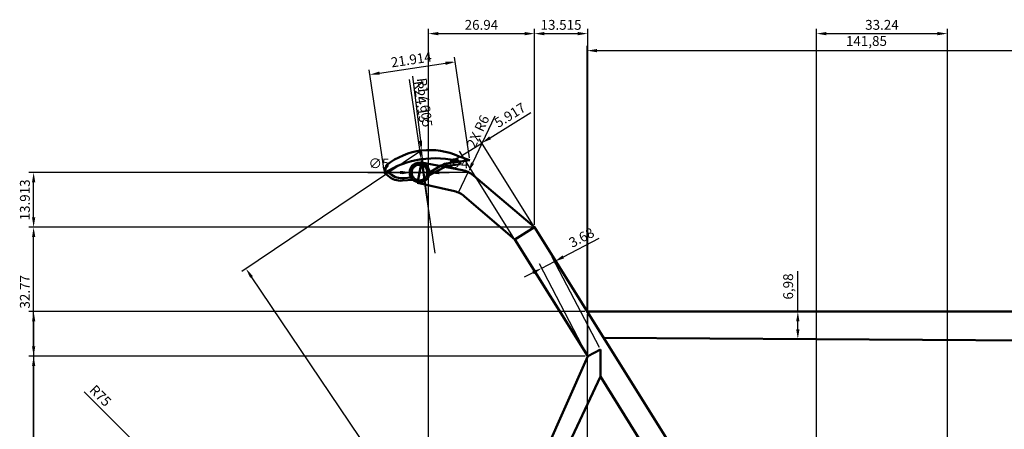
# Model space of a CAD drawing. Units: millimetres. Extents: x 1068 to 1546, y 1743 to 2032.
# Tile 5 of 9: x 1068 to 1318, y 1928 to 2032. Entities that reach past the tile are written whole.
import ezdxf

# ---------------------------------------------------------------- set-up
doc = ezdxf.new("R2010")
doc.units = ezdxf.units.MM
doc.layers.add('M-DIMS', color=2, linetype='Continuous', lineweight=25)
doc.layers.add('M-OUTL', color=7, linetype='Continuous', lineweight=50)
doc.styles.get("Standard").update_dxf_attribs({"font": 'arial.ttf'})
doc.dimstyles.new('ISO-25', dxfattribs={"dimtxt": 2.5, "dimasz": 2.5, "dimexe": 1.25, "dimexo": 0.625, "dimtad": 1, "dimtxsty": 'Standard', "dimcen": 2.5, "dimadec": 0, "dimazin": 0, "dimtfac": 1, "dimtmove": 0, "dimatfit": 3, "dimfxl": 1, "dimarcsym": 0})

# ---------------------------------------------------------------- blocks, each defined once
blk = doc.blocks.new('*D21')
at = {"layer": 'Defpoints', "color": 0, "transparency": 16777216}
for p in [(1266.05, 1957.56), (1267.8, 1957.56), (1267.8, 1950.59)]:
    blk.add_point(p, dxfattribs=at)
at = {"layer": 'M-DIMS', "color": 0, "lineweight": -2, "transparency": 16777216}
for p, q in [((1266.05, 1957.56), (1266.05, 1967.82)), ((1267.18, 1957.56), (1264.8, 1957.56)), ((1266.05, 1953.09), (1266.05, 1955.06)), ((1267.18, 1950.59), (1264.8, 1950.59))]:
    blk.add_line(p, q, dxfattribs=at)
at = {"layer": 'M-DIMS', "color": 0, "transparency": 16777216}
for points in [[(1265.63, 1955.06), (1266.47, 1955.06), (1266.05, 1957.56)], [(1265.63, 1953.09), (1266.47, 1953.09), (1266.05, 1950.59)]]:
    blk.add_solid(points, dxfattribs=at)
at = {"layer": 'M-DIMS', "color": 0, "transparency": 16777216, "insert": (1263.92, 1963.94), "char_height": 2.5, "attachment_point": 5, "rotation": 90}
blk.add_mtext('6,98', dxfattribs=at)
blk = doc.blocks.new('*D22')
at = {"layer": 'Defpoints', "color": 0, "transparency": 16777216}
for p in [(1354.41, 2023.87), (1212.56, 1957.56), (1354.41, 1957.56)]:
    blk.add_point(p, dxfattribs=at)
at = {"layer": 'M-DIMS', "color": 0, "lineweight": -2, "transparency": 16777216}
for p, q in [((1212.56, 1958.19), (1212.56, 2025.12)), ((1215.06, 2023.87), (1351.91, 2023.87)), ((1354.41, 1958.19), (1354.41, 2025.12))]:
    blk.add_line(p, q, dxfattribs=at)
at = {"layer": 'M-DIMS', "color": 0, "transparency": 16777216}
for points in [[(1215.06, 2024.29), (1215.06, 2023.46), (1212.56, 2023.87)], [(1351.91, 2024.29), (1351.91, 2023.46), (1354.41, 2023.87)]]:
    blk.add_solid(points, dxfattribs=at)
at = {"layer": 'M-DIMS', "color": 0, "transparency": 16777216, "insert": (1283.48, 2026), "char_height": 2.5, "attachment_point": 5}
blk.add_mtext('141,85', dxfattribs=at)
blk = doc.blocks.new('*D23')
at = {"layer": 'Defpoints', "color": 0, "transparency": 16777216}
for p in [(1170.51, 1998.5), (1125.92, 1968.44), (1270.79, 1849.76)]:
    blk.add_point(p, dxfattribs=at)
at = {"layer": 'M-DIMS', "color": 0, "lineweight": -2, "transparency": 16777216}
for p, q in [((1169.99, 1998.15), (1124.89, 1967.74)), ((1224.8, 1821.77), (1127.32, 1966.36)), ((1270.27, 1849.41), (1225.16, 1819))]:
    blk.add_line(p, q, dxfattribs=at)
at = {"layer": 'M-DIMS', "color": 0, "transparency": 16777216}
for points in [[(1127.67, 1966.6), (1126.98, 1966.13), (1125.92, 1968.44)], [(1225.15, 1822.01), (1224.45, 1821.54), (1226.2, 1819.7)]]:
    blk.add_solid(points, dxfattribs=at)
at = {"layer": 'M-DIMS', "color": 0, "transparency": 16777216, "insert": (1177.82, 1895.26), "char_height": 2.5, "attachment_point": 5, "rotation": 303.9872}
blk.add_mtext('179,38', dxfattribs=at)
blk = doc.blocks.new('*D26')
at = {"layer": 'Defpoints', "color": 0, "transparency": 16777216}
for p in [(1304.02, 2028.2), (1270.79, 1849.76), (1304.02, 1849.7)]:
    blk.add_point(p, dxfattribs=at)
at = {"layer": 'M-DIMS', "color": 0, "lineweight": -2, "transparency": 16777216}
for p, q in [((1270.79, 1850.39), (1270.79, 2029.45)), ((1273.29, 2028.2), (1301.52, 2028.2)), ((1304.02, 1850.33), (1304.02, 2029.45))]:
    blk.add_line(p, q, dxfattribs=at)
at = {"layer": 'M-DIMS', "color": 0, "transparency": 16777216}
for points in [[(1273.29, 2028.61), (1273.29, 2027.78), (1270.79, 2028.2)], [(1301.52, 2028.61), (1301.52, 2027.78), (1304.02, 2028.2)]]:
    blk.add_solid(points, dxfattribs=at)
at = {"layer": 'M-DIMS', "color": 0, "transparency": 16777216, "insert": (1287.41, 2030.1), "char_height": 2.5, "attachment_point": 5}
blk.add_mtext('33.24', dxfattribs=at)
blk = doc.blocks.new('*D28')
at = {"layer": 'Defpoints', "color": 0, "transparency": 16777216}
for p in [(1071.98, 1946.21), (1212.68, 1946.21), (1172.23, 1849.76)]:
    blk.add_point(p, dxfattribs=at)
at = {"layer": 'M-DIMS', "color": 0, "lineweight": -2, "transparency": 16777216}
for p, q in [((1212.06, 1946.21), (1070.73, 1946.21)), ((1071.98, 1852.26), (1071.98, 1943.71)), ((1171.6, 1849.76), (1070.73, 1849.76))]:
    blk.add_line(p, q, dxfattribs=at)
at = {"layer": 'M-DIMS', "color": 0, "transparency": 16777216}
for points in [[(1071.57, 1943.71), (1072.4, 1943.71), (1071.98, 1946.21)], [(1071.57, 1852.26), (1072.4, 1852.26), (1071.98, 1849.76)]]:
    blk.add_solid(points, dxfattribs=at)
at = {"layer": 'M-DIMS', "color": 0, "transparency": 16777216, "insert": (1070.08, 1897.98), "char_height": 2.5, "attachment_point": 5, "rotation": 90}
blk.add_mtext('96.44', dxfattribs=at)
blk = doc.blocks.new('*D29')
at = {"layer": 'Defpoints', "color": 0, "transparency": 16777216}
for p in [(1071.98, 1978.98), (1199.17, 1978.98), (1212.68, 1946.21)]:
    blk.add_point(p, dxfattribs=at)
at = {"layer": 'M-DIMS', "color": 0, "lineweight": -2, "transparency": 16777216}
for p, q in [((1198.54, 1978.98), (1070.73, 1978.98)), ((1071.98, 1948.71), (1071.98, 1976.48)), ((1212.06, 1946.21), (1070.73, 1946.21))]:
    blk.add_line(p, q, dxfattribs=at)
at = {"layer": 'M-DIMS', "color": 0, "transparency": 16777216}
for points in [[(1071.57, 1976.48), (1072.4, 1976.48), (1071.98, 1978.98)], [(1071.57, 1948.71), (1072.4, 1948.71), (1071.98, 1946.21)]]:
    blk.add_solid(points, dxfattribs=at)
at = {"layer": 'M-DIMS', "color": 0, "transparency": 16777216, "insert": (1070.08, 1962.59), "char_height": 2.5, "attachment_point": 5, "rotation": 90}
blk.add_mtext('32.77', dxfattribs=at)
blk = doc.blocks.new('*D30')
at = {"layer": 'Defpoints', "color": 0, "transparency": 16777216}
for p in [(1071.98, 1992.89), (1169.99, 1992.89), (1199.17, 1978.98)]:
    blk.add_point(p, dxfattribs=at)
at = {"layer": 'M-DIMS', "color": 0, "lineweight": -2, "transparency": 16777216}
for p, q in [((1169.36, 1992.89), (1070.73, 1992.89)), ((1071.98, 1981.48), (1071.98, 1990.39)), ((1198.54, 1978.98), (1070.73, 1978.98))]:
    blk.add_line(p, q, dxfattribs=at)
at = {"layer": 'M-DIMS', "color": 0, "transparency": 16777216}
for points in [[(1071.57, 1990.39), (1072.4, 1990.39), (1071.98, 1992.89)], [(1071.57, 1981.48), (1072.4, 1981.48), (1071.98, 1978.98)]]:
    blk.add_solid(points, dxfattribs=at)
at = {"layer": 'M-DIMS', "color": 0, "transparency": 16777216, "insert": (1070.08, 1985.94), "char_height": 2.5, "attachment_point": 5, "rotation": 90}
blk.add_mtext('13.913', dxfattribs=at)
blk = doc.blocks.new('*D31')
at = {"layer": 'Defpoints', "color": 0, "transparency": 16777216}
for p in [(1199.17, 2028.2), (1199.17, 1978.98), (1172.23, 1849.76)]:
    blk.add_point(p, dxfattribs=at)
at = {"layer": 'M-DIMS', "color": 0, "lineweight": -2, "transparency": 16777216}
for p, q in [((1172.23, 1850.39), (1172.23, 2029.45)), ((1174.73, 2028.2), (1196.67, 2028.2)), ((1199.17, 1979.6), (1199.17, 2029.45))]:
    blk.add_line(p, q, dxfattribs=at)
at = {"layer": 'M-DIMS', "color": 0, "transparency": 16777216}
for points in [[(1174.73, 2028.61), (1174.73, 2027.78), (1172.23, 2028.2)], [(1196.67, 2028.61), (1196.67, 2027.78), (1199.17, 2028.2)]]:
    blk.add_solid(points, dxfattribs=at)
at = {"layer": 'M-DIMS', "color": 0, "transparency": 16777216, "insert": (1185.7, 2030.1), "char_height": 2.5, "attachment_point": 5}
blk.add_mtext('26.94', dxfattribs=at)
blk = doc.blocks.new('*D32')
at = {"layer": 'Defpoints', "color": 0, "transparency": 16777216}
for p in [(1212.68, 2028.2), (1199.17, 1978.98), (1212.68, 1946.21)]:
    blk.add_point(p, dxfattribs=at)
at = {"layer": 'M-DIMS', "color": 0, "lineweight": -2, "transparency": 16777216}
for p, q in [((1199.17, 1979.6), (1199.17, 2029.45)), ((1201.67, 2028.2), (1210.18, 2028.2)), ((1212.68, 1946.83), (1212.68, 2029.45))]:
    blk.add_line(p, q, dxfattribs=at)
at = {"layer": 'M-DIMS', "color": 0, "transparency": 16777216}
for points in [[(1201.67, 2028.61), (1201.67, 2027.78), (1199.17, 2028.2)], [(1210.18, 2028.61), (1210.18, 2027.78), (1212.68, 2028.2)]]:
    blk.add_solid(points, dxfattribs=at)
at = {"layer": 'M-DIMS', "color": 0, "transparency": 16777216, "insert": (1205.92, 2030.1), "char_height": 2.5, "attachment_point": 5}
blk.add_mtext('13.515', dxfattribs=at)
blk = doc.blocks.new('*D33')
at = {"layer": 'Defpoints', "color": 0, "transparency": 16777216}
for p in [(1179.05, 2021.02), (1182.77, 1996.04), (1161.1, 1992.81)]:
    blk.add_point(p, dxfattribs=at)
at = {"layer": 'M-DIMS', "color": 0, "lineweight": -2, "transparency": 16777216}
for p, q in [((1159.84, 2018.15), (1176.57, 2020.65)), ((1182.68, 1996.66), (1178.86, 2022.25)), ((1161.01, 1993.43), (1157.19, 2019.02))]:
    blk.add_line(p, q, dxfattribs=at)
at = {"layer": 'M-DIMS', "color": 0, "transparency": 16777216}
for points in [[(1176.51, 2021.06), (1176.63, 2020.24), (1179.05, 2021.02)], [(1159.78, 2018.56), (1159.91, 2017.74), (1157.37, 2017.78)]]:
    blk.add_solid(points, dxfattribs=at)
at = {"layer": 'M-DIMS', "color": 0, "transparency": 16777216, "insert": (1167.93, 2021.28), "char_height": 2.5, "attachment_point": 5, "rotation": 8.4889}
blk.add_mtext('21.914', dxfattribs=at)
blk = doc.blocks.new('*D41')
at = {"layer": 'Defpoints', "color": 0, "transparency": 16777216}
for p in [(1185.78, 2000.39), (1199.17, 1978.98), (1194.15, 1975.84)]:
    blk.add_point(p, dxfattribs=at)
at = {"layer": 'M-DIMS', "color": 0, "lineweight": -2, "transparency": 16777216}
for p, q in [((1187.9, 2001.71), (1198.23, 2008.18)), ((1180.76, 1997.25), (1185.78, 2000.39)), ((1198.83, 1979.51), (1185.12, 2001.45)), ((1193.82, 1976.37), (1180.1, 1998.31)), ((1178.64, 1995.93), (1176.52, 1994.6))]:
    blk.add_line(p, q, dxfattribs=at)
at = {"layer": 'M-DIMS', "color": 0, "transparency": 16777216}
for points in [[(1187.68, 2002.07), (1188.12, 2001.36), (1185.78, 2000.39)], [(1178.42, 1996.28), (1178.86, 1995.57), (1180.76, 1997.25)]]:
    blk.add_solid(points, dxfattribs=at)
at = {"layer": 'M-DIMS', "color": 0, "transparency": 16777216, "insert": (1193.12, 2007.22), "char_height": 2.5, "attachment_point": 5, "rotation": 32.0179}
blk.add_mtext('5.917', dxfattribs=at)
blk = doc.blocks.new('*D44')
at = {"layer": 'Defpoints', "color": 0, "transparency": 16777216}
for p in [(1204.28, 1970.3), (1215.95, 1947.91), (1212.68, 1946.21)]:
    blk.add_point(p, dxfattribs=at)
at = {"layer": 'M-DIMS', "color": 0, "lineweight": -2, "transparency": 16777216}
for p, q in [((1206.5, 1971.46), (1215.58, 1976.19)), ((1215.66, 1948.46), (1203.7, 1971.41)), ((1212.39, 1946.76), (1200.43, 1969.71)), ((1201.01, 1968.6), (1204.28, 1970.3)), ((1198.79, 1967.44), (1196.58, 1966.29))]:
    blk.add_line(p, q, dxfattribs=at)
at = {"layer": 'M-DIMS', "color": 0, "transparency": 16777216}
for points in [[(1206.3, 1971.83), (1206.69, 1971.09), (1204.28, 1970.3)], [(1198.6, 1967.81), (1198.99, 1967.07), (1201.01, 1968.6)]]:
    blk.add_solid(points, dxfattribs=at)
at = {"layer": 'M-DIMS', "color": 0, "transparency": 16777216, "insert": (1211.27, 1976.09), "char_height": 2.5, "attachment_point": 5, "rotation": 27.5268}
blk.add_mtext('3.68', dxfattribs=at)
blk = doc.blocks.new('*D45')
at = {"layer": 'Defpoints', "color": 0, "transparency": 16777216}
for p in [(1212.56, 1957.56), (1273.55, 1860.03), (1273.55, 1744.51)]:
    blk.add_point(p, dxfattribs=at)
at = {"layer": 'M-DIMS', "color": 0, "lineweight": -2, "transparency": 16777216}
for p, q in [((1212.56, 1956.94), (1212.56, 1743.26)), ((1273.55, 1859.4), (1273.55, 1743.26)), ((1215.06, 1744.51), (1271.05, 1744.51))]:
    blk.add_line(p, q, dxfattribs=at)
at = {"layer": 'M-DIMS', "color": 0, "transparency": 16777216}
for points in [[(1215.06, 1744.93), (1215.06, 1744.1), (1212.56, 1744.51)], [(1271.05, 1744.93), (1271.05, 1744.1), (1273.55, 1744.51)]]:
    blk.add_solid(points, dxfattribs=at)
at = {"layer": 'M-DIMS', "color": 0, "transparency": 16777216, "insert": (1243.05, 1746.41), "char_height": 2.5, "attachment_point": 5}
blk.add_mtext('60.99', dxfattribs=at)
blk = doc.blocks.new('*D46')
at = {"layer": 'Defpoints', "color": 0, "transparency": 16777216}
for p in [(1212.56, 1957.56), (1071.98, 1860.03), (1273.55, 1860.03)]:
    blk.add_point(p, dxfattribs=at)
at = {"layer": 'M-DIMS', "color": 0, "lineweight": -2, "transparency": 16777216}
for p, q in [((1211.93, 1957.56), (1070.73, 1957.56)), ((1071.98, 1955.06), (1071.98, 1862.53)), ((1272.92, 1860.03), (1070.73, 1860.03))]:
    blk.add_line(p, q, dxfattribs=at)
at = {"layer": 'M-DIMS', "color": 0, "transparency": 16777216}
for points in [[(1071.57, 1955.06), (1072.4, 1955.06), (1071.98, 1957.56)], [(1071.57, 1862.53), (1072.4, 1862.53), (1071.98, 1860.03)]]:
    blk.add_solid(points, dxfattribs=at)
at = {"layer": 'M-DIMS', "color": 0, "transparency": 16777216, "insert": (1070.08, 1908.79), "char_height": 2.5, "attachment_point": 5, "rotation": 90}
blk.add_mtext('97.53', dxfattribs=at)
blk = doc.blocks.new('*D47')
at = {"layer": 'Defpoints', "color": 0, "transparency": 16777216}
for p in [(1361.34, 1946.14), (1282.2, 1868.65), (1361.34, 1744.51)]:
    blk.add_point(p, dxfattribs=at)
at = {"layer": 'M-DIMS', "color": 0, "lineweight": -2, "transparency": 16777216}
for p, q in [((1361.34, 1945.51), (1361.34, 1743.26)), ((1282.2, 1868.03), (1282.2, 1743.26)), ((1284.7, 1744.51), (1358.84, 1744.51))]:
    blk.add_line(p, q, dxfattribs=at)
at = {"layer": 'M-DIMS', "color": 0, "transparency": 16777216}
for points in [[(1284.7, 1744.93), (1284.7, 1744.1), (1282.2, 1744.51)], [(1358.84, 1744.93), (1358.84, 1744.1), (1361.34, 1744.51)]]:
    blk.add_solid(points, dxfattribs=at)
at = {"layer": 'M-DIMS', "color": 0, "transparency": 16777216, "insert": (1321.77, 1746.41), "char_height": 2.5, "attachment_point": 5}
blk.add_mtext('79.14', dxfattribs=at)
blk = doc.blocks.new('*D48')
at = {"layer": 'Defpoints', "color": 0, "transparency": 16777216}
for p in [(1361.34, 1946.14), (1507.48, 1946.14), (1282.2, 1868.65)]:
    blk.add_point(p, dxfattribs=at)
at = {"layer": 'M-DIMS', "color": 0, "lineweight": -2, "transparency": 16777216}
for p, q in [((1361.96, 1946.14), (1508.73, 1946.14)), ((1507.48, 1871.15), (1507.48, 1943.64)), ((1282.82, 1868.65), (1508.73, 1868.65))]:
    blk.add_line(p, q, dxfattribs=at)
at = {"layer": 'M-DIMS', "color": 0, "transparency": 16777216}
for points in [[(1507.06, 1943.64), (1507.89, 1943.64), (1507.48, 1946.14)], [(1507.06, 1871.15), (1507.89, 1871.15), (1507.48, 1868.65)]]:
    blk.add_solid(points, dxfattribs=at)
at = {"layer": 'M-DIMS', "color": 0, "transparency": 16777216, "insert": (1505.58, 1907.39), "char_height": 2.5, "attachment_point": 5, "rotation": 90}
blk.add_mtext('77.49', dxfattribs=at)
blk = doc.blocks.new('*D57')
at = {"layer": 'Defpoints', "color": 0, "transparency": 16777216}
for p in [(1119.2, 1902.8), (1172.23, 1849.76)]:
    blk.add_point(p, dxfattribs=at)
at = {"layer": 'M-DIMS', "color": 0, "lineweight": -2, "transparency": 16777216}
for p, q in [((1084.82, 1937.18), (1117.43, 1904.57)), ((1172.23, 1849.76), (1119.2, 1902.8))]:
    blk.add_line(p, q, dxfattribs=at)
at = {"layer": 'M-DIMS', "color": 0, "transparency": 16777216}
blk.add_solid([(1117.73, 1904.86), (1117.14, 1904.27), (1119.2, 1902.8)], dxfattribs=at)
at = {"layer": 'M-DIMS', "color": 0, "transparency": 16777216, "insert": (1088.72, 1935.96), "char_height": 2.5, "attachment_point": 5, "rotation": 314.9948}
blk.add_mtext('R75', dxfattribs=at)
blk = doc.blocks.new('*D65')
at = {"layer": 'Defpoints', "color": 0, "transparency": 16777216}
for p in [(1170.38, 1996.26), (1173.97, 1972.4)]:
    blk.add_point(p, dxfattribs=at)
at = {"layer": 'M-DIMS', "color": 0, "lineweight": -2, "transparency": 16777216}
for p, q in [((1167.32, 2016.55), (1170, 1998.73)), ((1173.97, 1972.4), (1170.38, 1996.26))]:
    blk.add_line(p, q, dxfattribs=at)
at = {"layer": 'M-DIMS', "color": 0, "transparency": 16777216}
blk.add_solid([(1170.42, 1998.79), (1169.59, 1998.67), (1170.38, 1996.26)], dxfattribs=at)
at = {"layer": 'M-DIMS', "color": 0, "transparency": 16777216, "insert": (1170.1, 2010.86), "char_height": 2.5, "attachment_point": 5, "rotation": 278.5724}
blk.add_mtext('R24.13', dxfattribs=at)
blk = doc.blocks.new('*D66')
at = {"layer": 'Defpoints', "color": 0, "transparency": 16777216}
for p in [(1170.51, 1998.5), (1172.63, 1981.02)]:
    blk.add_point(p, dxfattribs=at)
at = {"layer": 'M-DIMS', "color": 0, "lineweight": -2, "transparency": 16777216}
for p, q in [((1168.22, 2017.4), (1170.21, 2000.98)), ((1172.63, 1981.02), (1170.51, 1998.5))]:
    blk.add_line(p, q, dxfattribs=at)
at = {"layer": 'M-DIMS', "color": 0, "transparency": 16777216}
blk.add_solid([(1170.63, 2001.03), (1169.8, 2000.93), (1170.51, 1998.5)], dxfattribs=at)
at = {"layer": 'M-DIMS', "color": 0, "transparency": 16777216, "insert": (1170.95, 2010.66), "char_height": 2.5, "attachment_point": 5, "rotation": 276.9175}
blk.add_mtext('R17.605', dxfattribs=at)
blk = doc.blocks.new('*D76')
at = {"layer": 'Defpoints', "color": 0, "transparency": 16777216}
for p in [(1182.37, 1993.03), (1179.78, 1987.62)]:
    blk.add_point(p, dxfattribs=at)
at = {"layer": 'M-DIMS', "color": 0, "lineweight": -2, "transparency": 16777216}
for p, q in [((1189.13, 2007.19), (1183.44, 1995.29)), ((1179.78, 1987.62), (1182.37, 1993.03))]:
    blk.add_line(p, q, dxfattribs=at)
at = {"layer": 'M-DIMS', "color": 0, "transparency": 16777216}
blk.add_solid([(1183.07, 1995.47), (1183.82, 1995.11), (1182.37, 1993.03)], dxfattribs=at)
at = {"layer": 'M-DIMS', "color": 0, "transparency": 16777216, "insert": (1185.11, 2003.19), "char_height": 2.5, "attachment_point": 5, "rotation": 64.4837}
blk.add_mtext('2X R6', dxfattribs=at)
blk = doc.blocks.new('*D79')
at = {"layer": 'Defpoints', "color": 0, "transparency": 16777216}
for p in [(1167.49, 1992.9), (1172.49, 1992.89)]:
    blk.add_point(p, dxfattribs=at)
at = {"layer": 'M-DIMS', "color": 0, "lineweight": -2, "transparency": 16777216}
for p, q in [((1156.86, 1992.93), (1164.99, 1992.91)), ((1172.49, 1992.89), (1167.49, 1992.9)), ((1174.99, 1992.88), (1177.49, 1992.87))]:
    blk.add_line(p, q, dxfattribs=at)
at = {"layer": 'M-DIMS', "color": 0, "transparency": 16777216}
for points in [[(1164.99, 1993.32), (1164.98, 1992.49), (1167.49, 1992.9)], [(1174.99, 1993.29), (1174.98, 1992.46), (1172.49, 1992.89)]]:
    blk.add_solid(points, dxfattribs=at)
at = {"layer": 'M-DIMS', "color": 0, "transparency": 16777216, "insert": (1159.68, 1994.89), "char_height": 2.5, "attachment_point": 5, "rotation": 359.8328}
blk.add_mtext('∅5', dxfattribs=at)
blk = doc.blocks.new('*D80')
at = {"layer": 'Defpoints', "color": 0, "transparency": 16777216}
for p in [(1167.99, 1992.89), (1171.99, 1992.9)]:
    blk.add_point(p, dxfattribs=at)
at = {"layer": 'M-DIMS', "color": 0, "lineweight": -2, "transparency": 16777216}
for p, q in [((1165.49, 1992.88), (1162.99, 1992.87)), ((1167.99, 1992.89), (1171.99, 1992.9)), ((1182.58, 1992.94), (1174.49, 1992.91))]:
    blk.add_line(p, q, dxfattribs=at)
at = {"layer": 'M-DIMS', "color": 0, "transparency": 16777216}
for points in [[(1165.48, 1993.29), (1165.49, 1992.46), (1167.99, 1992.89)], [(1174.48, 1993.33), (1174.49, 1992.49), (1171.99, 1992.9)]]:
    blk.add_solid(points, dxfattribs=at)
at = {"layer": 'M-DIMS', "color": 0, "transparency": 16777216, "insert": (1179.78, 1994.9), "char_height": 2.5, "attachment_point": 5, "rotation": 0.2063}
blk.add_mtext('∅4', dxfattribs=at)

msp = doc.modelspace()

# ---------------------------------------------------------------- linework, layer by layer
at = {"layer": 'M-OUTL'}
for p, q in [((1169.5051, 1990.3234), (1170.4659, 1995.4621)), ((1180.8842, 1993.5142), (1170.4486, 1995.4653)), ((1177.3514, 1995.2964), (1180.2594, 1995.6971)), ((1182.7731, 1996.0435), (1180.0358, 1996.9929)), ((1180.2594, 1995.6971), (1182.7731, 1996.0435)), ((1180.2594, 1995.6971), (1180.3491, 1995.0462)), ((1161.0994, 1992.8087), (1161.6258, 1994.7591)), ((1161.7904, 1993.15), (1161.0994, 1992.8087)), ((1162.5033, 1992.5661), (1161.7904, 1993.15)), ((1176.1114, 1994.1402), (1172.3597, 1992.1098)), ((1172.4855, 1992.8927), (1175.5122, 1994.6606)), ((1180.3491, 1995.0462), (1177.8086, 1994.6961)), ((1162.0058, 1992.028), (1161.0994, 1992.8087)), ((1168.3037, 1991.043), (1165.6669, 1990.8324)), ((1167.8411, 1991.6077), (1166.1159, 1991.4538)), ((1168.3037, 1991.043), (1168.3037, 1991.043)), ((1199.166, 1978.9798), (1183.6733, 1992.1831)), ((1178.8506, 1988.1569), (1169.5051, 1990.3234)), ((1194.1495, 1975.8429), (1181.4201, 1986.8504)), ((1194.1495, 1975.8429), (1199.166, 1978.9798)), ((1272.1243, 1862.3034), (1199.166, 1978.9798)), ((1212.6811, 1946.2068), (1194.1495, 1975.8429)), ((1212.5594, 1957.5607), (1352.9598, 1957.5607)), ((1216.7245, 1950.8999), (1358.9799, 1950.024)), ((1212.6811, 1946.2068), (1215.9477, 1947.9092)), ((1215.9477, 1947.9092), (1215.8973, 1941.0634)), ((1172.2281, 1854.7623), (1212.6811, 1946.2068)), ((1175.1069, 1853.8504), (1215.8973, 1941.0634)), ((1267.1078, 1859.1666), (1215.8973, 1941.0634))]:
    msp.add_line(p, q, dxfattribs=at)
for radius in [2.5, 2]:
    msp.add_circle((1169.9855, 1992.8927), radius, dxfattribs=at)
for centre, radius, start, end in [((1172.6334, 1981.0199), 17.6049, 65.135339, 128.701171), ((1173.9735, 1972.4028), 24.1276, 74.898415, 122.247726), ((1178.034, 1990.3432), 5, 97.846481, 120.289159), ((1178.4912, 1989.7429), 5, 97.846481, 118.422502), ((1179.7815, 1987.6164), 6, 49.561476, 79.410191), ((1165.2688, 1995.8165), 5, 229.261161, 274.566457), ((1165.6717, 1996.434), 5, 230.677883, 275.0965), ((1177.4956, 1982.3119), 6, 49.149097, 76.947629)]:
    msp.add_arc(centre, radius, start, end, dxfattribs=at)

# ---------------------------------------------------------------- dimensions: what is measured, and where the dimension line sits
at = {"layer": 'M-DIMS'}
for base, p1, p2, override, picture, middle in [((1199.166, 2028.1976), (1172.2281, 1849.7623), (1199.166, 1978.9798), {"dimdec": 2, "dimlfac": 1, "dimrnd": 0, "dimzin": 0, "dimdsep": 46, "dimlunit": 2}, '*D31', (1185.697, 2030.099)), ((1212.6811, 2028.1976), (1199.166, 1978.9798), (1212.6811, 1946.2068), {"dimdec": 3, "dimlfac": 1, "dimrnd": 0, "dimzin": 0, "dimdsep": 46, "dimlunit": 2}, '*D32', (1205.9235, 2030.0999)), ((1304.0238, 2028.1976), (1270.787, 1849.7623), (1304.0238, 1849.7019), {"dimdec": 2, "dimlfac": 1, "dimrnd": 0, "dimzin": 0, "dimdsep": 46, "dimlunit": 2}, '*D26', (1287.4054, 2030.0999)), ((1354.405, 2023.8738), (1212.5594, 1957.5607), (1354.405, 1957.5607), {"dimclrd": 0, "dimclre": 0, "dimclrt": 0}, '*D22', (1283.4822, 2026.0012)), ((1273.5484, 1744.5123), (1212.5594, 1957.5607), (1273.5484, 1860.0259), {"dimdec": 2, "dimlfac": 1, "dimrnd": 0, "dimzin": 0, "dimdsep": 46, "dimlunit": 2}, '*D45', (1243.0539, 1746.4138)), ((1361.339, 1744.5123), (1282.1954, 1868.6519), (1361.339, 1946.1377), {"dimdec": 2, "dimlfac": 1, "dimrnd": 0, "dimzin": 0, "dimdsep": 46, "dimlunit": 2}, '*D47', (1321.7672, 1746.4138))]:
    dim = msp.add_linear_dim(base=base, p1=p1, p2=p2, dimstyle='ISO-25', override=override, dxfattribs=at)
    dim.commit()
    dim.dimension.update_dxf_attribs({"geometry": picture, "text_midpoint": middle})
for base, p1, p2, angle, override, picture, middle in [((1179.0457, 2021.0169), (1161.0994, 1992.8087), (1182.7731, 1996.0435), 8.48894, {"dimdec": 3, "dimlfac": 1, "dimrnd": 0, "dimzin": 0, "dimdsep": 46, "dimlunit": 2}, '*D33', (1167.9282, 2021.2801)), ((1185.7788, 2000.3888), (1194.1495, 1975.8429), (1199.166, 1978.9798), 32.017948, {"dimdec": 3, "dimlfac": 1, "dimrnd": 0, "dimzin": 0, "dimdsep": 46, "dimlunit": 2}, '*D41', (1193.1165, 2007.2197)), ((1071.9839, 1992.8927), (1199.166, 1978.9798), (1169.9855, 1992.8927), 90, {"dimdec": 3, "dimlfac": 1, "dimrnd": 0, "dimzin": 0, "dimdsep": 46, "dimlunit": 2}, '*D30', (1070.0816, 1985.9363)), ((1071.9839, 1978.9798), (1212.6811, 1946.2068), (1199.166, 1978.9798), 90, {"dimdec": 2, "dimlfac": 1, "dimrnd": 0, "dimzin": 0, "dimdsep": 46, "dimlunit": 2}, '*D29', (1070.0816, 1962.5933)), ((1204.278, 1970.3007), (1212.6811, 1946.2068), (1215.9477, 1947.9092), 27.526816, {"dimdec": 2, "dimlfac": 1, "dimrnd": 0, "dimzin": 0, "dimdsep": 46, "dimlunit": 2}, '*D44', (1211.268, 1976.0888)), ((1266.0489, 1957.5607), (1267.8046, 1950.5854), (1267.8046, 1957.5607), 90, {"dimclrd": 0, "dimclre": 0, "dimclrt": 0}, '*D21', (1263.9215, 1963.9421)), ((1071.9839, 1860.0259), (1212.5594, 1957.5607), (1273.5484, 1860.0259), 90, {"dimdec": 2, "dimlfac": 1, "dimrnd": 0, "dimzin": 0, "dimdsep": 46, "dimlunit": 2}, '*D46', (1070.0816, 1908.7933)), ((1071.9839, 1946.2068), (1172.2281, 1849.7623), (1212.6811, 1946.2068), 90, {"dimdec": 2, "dimlfac": 1, "dimrnd": 0, "dimzin": 0, "dimdsep": 46, "dimlunit": 2}, '*D28', (1070.0825, 1897.9845)), ((1507.4781, 1946.1377), (1282.1954, 1868.6519), (1361.339, 1946.1377), 90, {"dimdec": 2, "dimlfac": 1, "dimrnd": 0, "dimzin": 0, "dimdsep": 46, "dimlunit": 2}, '*D48', (1505.5767, 1907.3948))]:
    dim = msp.add_linear_dim(base=base, p1=p1, p2=p2, angle=angle, dimstyle='ISO-25', override=override, dxfattribs=at)
    dim.commit()
    dim.dimension.update_dxf_attribs({"geometry": picture, "text_midpoint": middle})
for center, mpoint, override, picture, middle in [((1173.9735, 1972.4028), (1170.377, 1996.2608), {"dimdec": 2, "dimlfac": 1, "dimrnd": 0, "dimzin": 0, "dimdsep": 46, "dimlunit": 2}, '*D65', (1168.2192, 2010.5756)), ((1172.2281, 1849.7623), (1119.1999, 1902.8001), {"dimdec": 0, "dimlfac": 1, "dimrnd": 0, "dimzin": 0, "dimdsep": 46, "dimlunit": 2}, '*D57', (1087.383, 1934.6228))]:
    dim = msp.add_radius_dim(center=center, mpoint=mpoint, dimstyle='ISO-25', override=override, dxfattribs=at)
    dim.commit()
    dim.dimension.update_dxf_attribs({"geometry": picture, "text_midpoint": middle, "dimtype": 164})
dim = msp.add_radius_dim(center=(1172.6334, 1981.0199), mpoint=(1170.513, 1998.4967), dimstyle='ISO-25', override={"dimdec": 3, "dimlfac": 1, "dimrnd": 0, "dimzin": 0, "dimdsep": 46, "dimlunit": 2}, dxfattribs=at)
dim.commit()
dim.dimension.update_dxf_attribs({"geometry": '*D66', "text_midpoint": (1170.9529, 2010.6581)})
dim = msp.add_radius_dim(center=(1179.7815, 1987.6164), mpoint=(1182.3661, 1993.0312), text='2X <>', dimstyle='ISO-25', override={"dimdec": 0, "dimlfac": 1, "dimrnd": 0, "dimzin": 0, "dimdsep": 46, "dimlunit": 2}, dxfattribs=at)
dim.commit()
dim.dimension.update_dxf_attribs({"geometry": '*D76', "text_midpoint": (1185.1073, 2003.1881)})
dim = msp.add_aligned_dim(p1=(1270.787, 1849.7623), p2=(1170.5128, 1998.4966), distance=53.7765, dimstyle='ISO-25', override={"dimclrd": 0, "dimclre": 0, "dimclrt": 0}, dxfattribs=at)
dim.commit()
dim.dimension.update_dxf_attribs({"geometry": '*D23', "text_midpoint": (1177.8244, 1895.2572)})
dim = msp.add_diameter_dim_2p(p1=(1172.4855, 1992.8854), p2=(1167.4855, 1992.9), dimstyle='ISO-25', override={"dimdec": 0, "dimlfac": 1, "dimrnd": 0, "dimzin": 0, "dimdsep": 46, "dimlunit": 2}, dxfattribs=at)
dim.commit()
dim.dimension.update_dxf_attribs({"geometry": '*D79', "text_midpoint": (1159.6718, 1992.9228), "dimtype": 163})
dim = msp.add_diameter_dim_2p(p1=(1167.9855, 1992.8855), p2=(1171.9855, 1992.8999), dimstyle='ISO-25', override={"dimdec": 0, "dimlfac": 1, "dimrnd": 0, "dimzin": 0, "dimdsep": 46, "dimlunit": 2}, dxfattribs=at)
dim.commit()
dim.dimension.update_dxf_attribs({"geometry": '*D80', "text_midpoint": (1179.7847, 1992.928)})

doc.saveas('drawing.dxf')
